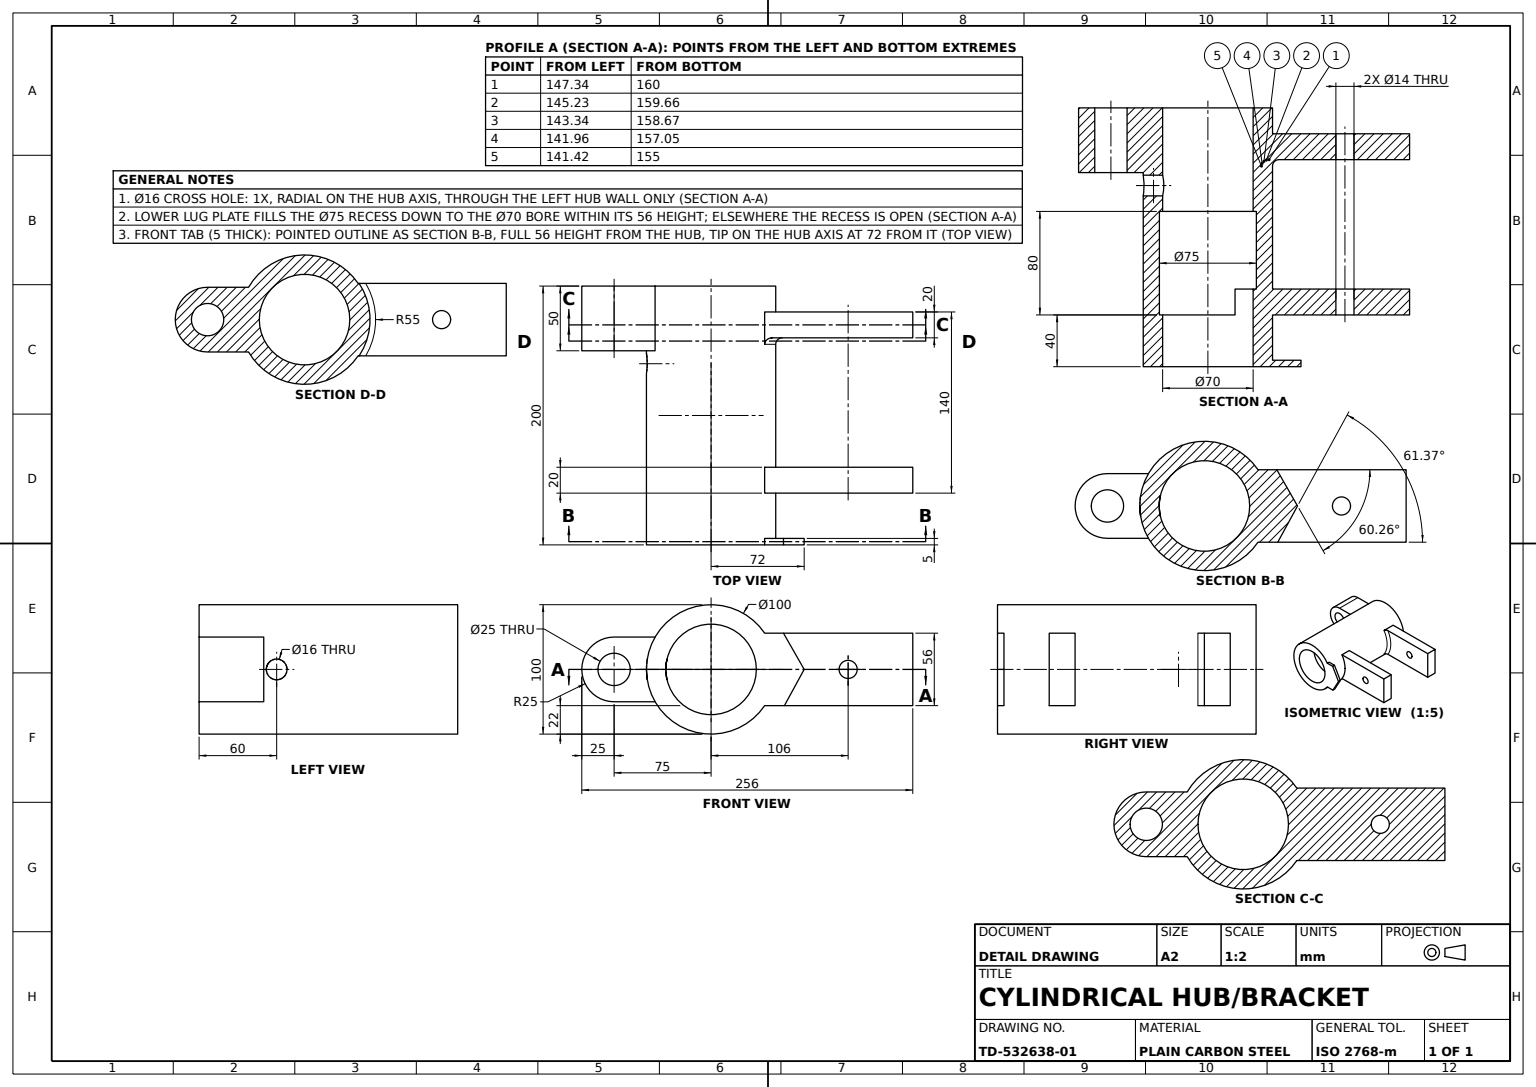
SolidWorks part; units mm, degrees
material "Plain Carbon Steel"
ref_plane "Front Plane" through (0, 0, 0) normal (0, 0, 1) x (1, 0, 0)
ref_plane "Top Plane" through (0, 0, 0) normal (0, 1, 0) x (1, 0, 0)
ref_plane "Right Plane" through (0, 0, 0) normal (1, 0, 0) x (0, 0, -1)
sketch "Body Profile Ø100" plane through (0, 0, 0) normal (0, 0, 1) x (1, 0, 0)
  circle A0 centre (0, 0) radius 50
  dimension "D1" = 100
extrude "Housing Body Ø100x200" add sketch "Body Profile Ø100" along normal blind 200
sketch "Front Bore Profile Ø70" plane through (0, 0, 200) normal (0, 0, 1) x (1, 0, 0)
  circle A0 centre (0, 0) radius 35
  dimension "D1" = 70
extrude "Front Bore Ø70x40" cut sketch "Front Bore Profile Ø70" against normal blind 40
sketch "Inner Recess Profile Ø75" plane through (0, 0, 160) normal (0, 0, 1) x (1, 0, 0)
  circle A0 centre (0, 0) radius 37.5
  dimension "D1" = 75
extrude "Inner Recess Ø75x80" cut sketch "Inner Recess Profile Ø75" against normal blind 80
sketch "Through Bore Profile Ø70" plane through (0, 0, 0) normal (0, 0, -1) x (-1, 0, 0)
  circle A0 centre (0, 0) radius 35
  dimension "D1" = 70
extrude "Through Bore Ø70" cut sketch "Through Bore Profile Ø70" against normal through all
ref_plane "Plane1" through (0, 0, 200) normal (0, 0, 1) x (1, 0, 0)
sketch "Rear Tab Profile" plane through (0, 0, 200) normal (0, 0, 1) x (1, 0, 0)
  line L0 (56, 28) -> (72, 0)
  line L3 (56.7123, -28) -> (72, 0)
  line L4 (56, 28) -> (41.4246, 28)
  line L5 (41.4246, 28) -> (56, 28)
  line L8 (56.7123, -28) -> (41.4246, -28)
  arc A0 (0, -50) -> (41.4246, 28) centre (0, 0) ccw
  circle A1 centre (0, 0) radius 50 construction
  point P7 (72, 50)
  point P9 (72, -50)
  dimension "D1" = 14.5754
  dimension "D4" = 72
  dimension "D2" = 15.2877
  dimension "D3" = 56
  dimension "D5" = 28
  dimension "D6" = 28
extrude "Rear Tab 5mm" add sketch "Rear Tab Profile" against normal blind 5 contours A0 L8 L3 L0 L4
ref_plane "Plane2" through (0, 0, 140) normal (0, 0, 1) x (1, 0, 0)
sketch "Lug Plates Profile" plane through (0, 0, 140) normal (0, 0, 1) x (1, 0, 0)
  line L0 (0, 0) -> (156, 0) construction
  line L1 (21, -28) -> (156, -28)
  line L2 (21, 28) -> (156, 28)
  line L3 (156, 28) -> (156, -28)
  line L5 (0, 28) -> (156, 28) construction
  line L6 (0, -28) -> (156, -28) construction
  arc A0 (21, -28) -> (21, 28) centre (0, 0) ccw
  dimension "D4" = 70
  dimension "D1" = 156
  dimension "D2" = 28
  dimension "D3" = 28
extrude "Lug Plates" add sketch "Lug Plates Profile" along normal blind 20
ref_plane "Plane3" through (0, 0, 20) normal (0, 0, 1) x (1, 0, 0)
sketch "Lug Web Profile" plane through (0, 0, 20) normal (0, 0, 1) x (1, 0, 0)
  line L0 (41.4246, 28) -> (156, 28)
  line L1 (156, 28) -> (156, -28)
  line L2 (156, -28) -> (41.4246, -28)
  line L3 (41.4246, -28) -> (41.4246, 28)
extrude "Lug Web" add sketch "Lug Web Profile" along normal blind 20
sketch "Lug Pin Holes Profile Ø14" plane through (0, 0, 160) normal (0, 0, 1) x (1, 0, 0)
  line L0 (0, 0) -> (106, 0) construction
  circle A0 centre (106, 0) radius 7
  dimension "D1" = 14
  dimension "D2" = 106
extrude "Lug Pin Holes Ø14" cut sketch "Lug Pin Holes Profile Ø14" against normal through all
fillet "Lug Web Fillet R5" radius 5 1 edges at (50, 0, 40)
ref_plane "Plane4" through (0, 0, 0) normal (0, 0, 1) x (1, 0, 0)
sketch "Top Boss Profile" plane through (0, 0, 0) normal (0, 0, 1) x (1, 0, 0)
  line L0 (-50, 0) -> (-75, 0) construction
  line L1 (-75, 25) -> (-43.3013, 25)
  line L2 (-75, -25) -> (-43.3013, -25)
  arc A0 (41.4246, 28) -> (41.4246, -28) centre (0, 0) ccw construction
  arc A1 (-75, 25) -> (-75, -25) centre (-75, 0) ccw
  circle A2 centre (-75, 0) radius 12.5
  arc A3 (-43.3013, 25) -> (-43.3013, -25) centre (0, 0) ccw
  dimension "D1" = 50
  dimension "D2" = 25
  dimension "D3" = 50
  dimension "D4" = 25
extrude "Top Boss" add sketch "Top Boss Profile" along normal blind 50
ref_plane "Plane5" through (-50, 0, 0) normal (1, 0, 0) x (0, 0, -1)
sketch "Top Boss Hole Profile Ø16" plane through (-50, 0, 0) normal (1, 0, 0) x (0, 0, -1)
  line L0 (0, 0) -> (-60, 0) construction
  line L1 (0, -25) -> (0, 25) construction
  circle A0 centre (-60, 0) radius 8
  dimension "D1" = 16
  dimension "D2" = 60
extrude "Top Boss Hole Ø16" cut sketch "Top Boss Hole Profile Ø16" along normal blind 50
